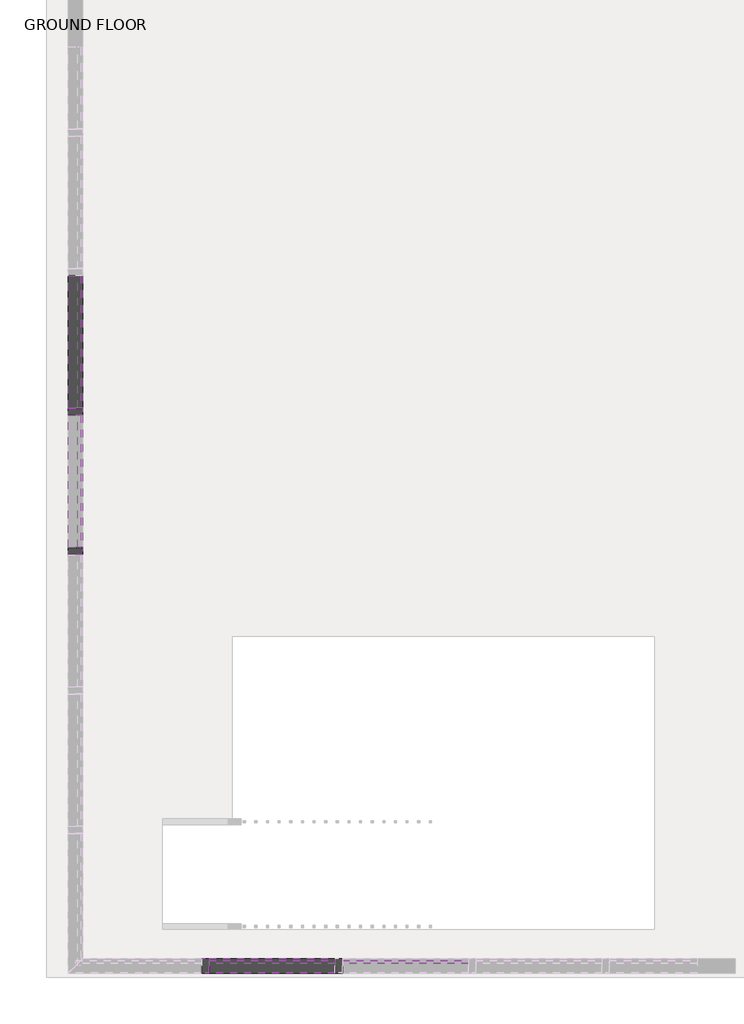
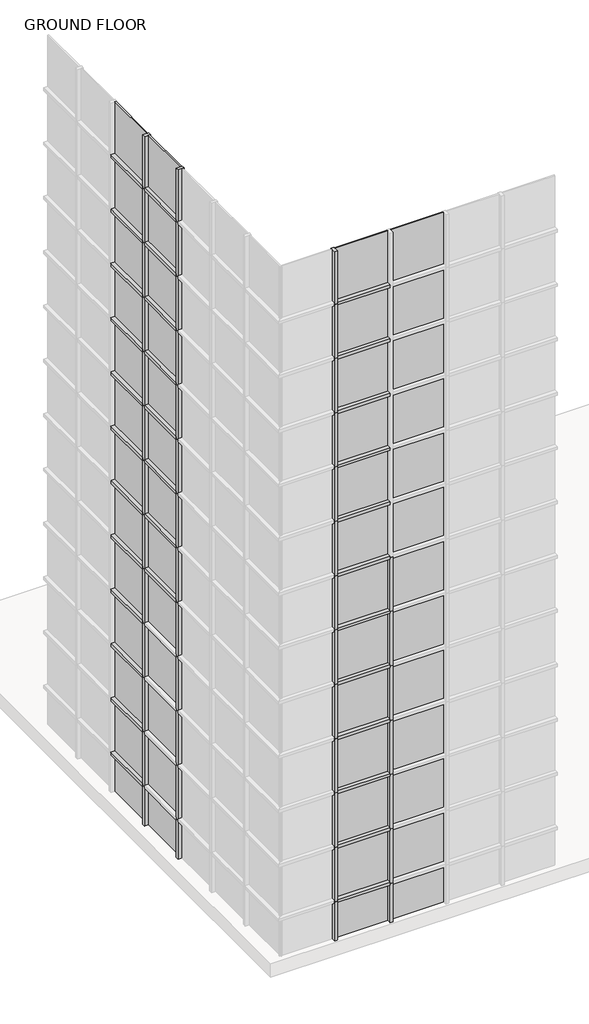
# One storey, part 2 of 16: 78 members, 52 plates.
"""IFC4 building model written with IfcOpenShell, lengths in millimetres."""

from ifc_helpers import new_model, si_unit, origin, place, context, project, spatial, transform, mapped, element, save
from components import member_d518c94e, member_b860638c, member_31fee25f, member_49b1bc66, system_panel_glazed_5cba32e5, system_panel_glazed_49652e9e

model = new_model("IFC4")

# Units and contexts
model_context = context("Model", 3, world=origin())
ifc_project = project(units=[si_unit("LENGTHUNIT", "METRE", prefix="MILLI")], contexts=[model_context])

# Site, building, storey
site = spatial("IfcSite", under=ifc_project)
building = spatial("IfcBuilding", under=site)
storey = spatial("IfcBuildingStorey", under=building, Name="GROUND FLOOR", Elevation=0.0)

# Members
placement = place(None, origin())
member_shape = member_d518c94e(model_context)
element("IfcMember", 1, ObjectType="Rectangular Mullion : 2.5\" x 5\" rectangular", at=placement, inside=storey, context=model_context, shape_type="MappedRepresentation", body=[
    mapped(member_shape, transform((-6857.4632917, -5739.2238032, 1168.8884615), x_axis=(0.0, 0.0, 1.0), y_axis=(0.0, -1.0, 0.0), z_axis=(1.0, 0.0, 0.0))),
])
element("IfcMember", 2, ObjectType="Rectangular Mullion : 2.5\" x 5\" rectangular", at=placement, inside=storey, context=model_context, shape_type="MappedRepresentation", body=[
    mapped(member_shape, transform((-6857.4632917, -5739.2238032, 2369.5269231), x_axis=(0.0, 0.0, 1.0), y_axis=(0.0, -1.0, 0.0), z_axis=(1.0, 0.0, 0.0))),
])
element("IfcMember", 3, ObjectType="Rectangular Mullion : 2.5\" x 5\" rectangular", at=placement, inside=storey, context=model_context, shape_type="MappedRepresentation", body=[
    mapped(member_shape, transform((-6857.4632917, -5739.2238032, 3570.1653846), x_axis=(0.0, 0.0, 1.0), y_axis=(0.0, -1.0, 0.0), z_axis=(1.0, 0.0, 0.0))),
])
element("IfcMember", 4, ObjectType="Rectangular Mullion : 2.5\" x 5\" rectangular", at=placement, inside=storey, context=model_context, shape_type="MappedRepresentation", body=[
    mapped(member_shape, transform((-6857.4632917, -5739.2238032, 4770.8038462), x_axis=(0.0, 0.0, 1.0), y_axis=(0.0, -1.0, 0.0), z_axis=(1.0, 0.0, 0.0))),
])
element("IfcMember", 5, ObjectType="Rectangular Mullion : 2.5\" x 5\" rectangular", at=placement, inside=storey, context=model_context, shape_type="MappedRepresentation", body=[
    mapped(member_shape, transform((-6857.4632917, -5739.2238032, 5971.4423077), x_axis=(0.0, 0.0, 1.0), y_axis=(0.0, -1.0, 0.0), z_axis=(1.0, 0.0, 0.0))),
])
element("IfcMember", 6, ObjectType="Rectangular Mullion : 2.5\" x 5\" rectangular", at=placement, inside=storey, context=model_context, shape_type="MappedRepresentation", body=[
    mapped(member_shape, transform((-6857.4632917, -5739.2238032, 7172.0807692), x_axis=(0.0, 0.0, 1.0), y_axis=(0.0, -1.0, 0.0), z_axis=(1.0, 0.0, 0.0))),
])
element("IfcMember", 7, ObjectType="Rectangular Mullion : 2.5\" x 5\" rectangular", at=placement, inside=storey, context=model_context, shape_type="MappedRepresentation", body=[
    mapped(member_shape, transform((-6857.4632917, -5739.2238032, 8372.7192308), x_axis=(0.0, 0.0, 1.0), y_axis=(0.0, -1.0, 0.0), z_axis=(1.0, 0.0, 0.0))),
])
element("IfcMember", 8, ObjectType="Rectangular Mullion : 2.5\" x 5\" rectangular", at=placement, inside=storey, context=model_context, shape_type="MappedRepresentation", body=[
    mapped(member_shape, transform((-6857.4632917, -5739.2238032, 9573.3576923), x_axis=(0.0, 0.0, 1.0), y_axis=(0.0, -1.0, 0.0), z_axis=(1.0, 0.0, 0.0))),
])
element("IfcMember", 9, ObjectType="Rectangular Mullion : 2.5\" x 5\" rectangular", at=placement, inside=storey, context=model_context, shape_type="MappedRepresentation", body=[
    mapped(member_shape, transform((-6857.4632917, -5739.2238032, 10773.9961538), x_axis=(0.0, 0.0, 1.0), y_axis=(0.0, -1.0, 0.0), z_axis=(1.0, 0.0, 0.0))),
])
element("IfcMember", 10, ObjectType="Rectangular Mullion : 2.5\" x 5\" rectangular", at=placement, inside=storey, context=model_context, shape_type="MappedRepresentation", body=[
    mapped(member_shape, transform((-6857.4632917, -5739.2238032, 11974.6346154), x_axis=(0.0, 0.0, 1.0), y_axis=(0.0, -1.0, 0.0), z_axis=(1.0, 0.0, 0.0))),
])
element("IfcMember", 11, ObjectType="Rectangular Mullion : 2.5\" x 5\" rectangular", at=placement, inside=storey, context=model_context, shape_type="MappedRepresentation", body=[
    mapped(member_shape, transform((-6857.4632917, -5739.2238032, 13175.2730769), x_axis=(0.0, 0.0, 1.0), y_axis=(0.0, -1.0, 0.0), z_axis=(1.0, 0.0, 0.0))),
])
element("IfcMember", 12, ObjectType="Rectangular Mullion : 2.5\" x 5\" rectangular", at=placement, inside=storey, context=model_context, shape_type="MappedRepresentation", body=[
    mapped(member_shape, transform((-6857.4632917, -5739.2238032, 14375.9115385), x_axis=(0.0, 0.0, 1.0), y_axis=(0.0, -1.0, 0.0), z_axis=(1.0, 0.0, 0.0))),
])
member_2_shape = member_b860638c(model_context)
element("IfcMember", 13, ObjectType="Rectangular Mullion : 2.5\" x 5\" rectangular", at=placement, inside=storey, context=model_context, shape_type="MappedRepresentation", body=[
    mapped(member_2_shape, transform((-7991.1825224, -5739.2238032, 0.0), x_axis=(1.0, 0.0, 0.0), y_axis=(0.0, -1.0, 0.0), z_axis=(0.0, 0.0, -1.0))),
])
element("IfcMember", 14, ObjectType="Rectangular Mullion : 2.5\" x 5\" rectangular", at=placement, inside=storey, context=model_context, shape_type="MappedRepresentation", body=[
    mapped(member_2_shape, transform((-6825.7132917, -5739.2238032, 0.0), x_axis=(1.0, 0.0, 0.0), y_axis=(0.0, -1.0, 0.0), z_axis=(0.0, 0.0, -1.0))),
])
element("IfcMember", 15, ObjectType="Rectangular Mullion : 2.5\" x 5\" rectangular", at=placement, inside=storey, context=model_context, shape_type="MappedRepresentation", body=[
    mapped(member_2_shape, transform((-9124.9017534, -901.7938032, 0.0), x_axis=(0.0, -1.0, 0.0), y_axis=(-1.0, 0.0, 0.0), z_axis=(0.0, 0.0, -1.0))),
])
element("IfcMember", 16, ObjectType="Rectangular Mullion : 2.5\" x 5\" rectangular", at=placement, inside=storey, context=model_context, shape_type="MappedRepresentation", body=[
    mapped(member_2_shape, transform((-9124.9017534, -2119.0888031, 0.0), x_axis=(0.0, -1.0, 0.0), y_axis=(-1.0, 0.0, 0.0), z_axis=(0.0, 0.0, -1.0))),
])
member_3_shape = member_31fee25f(model_context)
element("IfcMember", 17, ObjectType="Rectangular Mullion : 2.5\" x 5\" rectangular", at=placement, inside=storey, context=model_context, shape_type="MappedRepresentation", body=[
    mapped(member_3_shape, transform((-7991.1825224, -5739.2238032, 1168.8884615), x_axis=(1.0, 0.0, 0.0), y_axis=(0.0, -1.0, 0.0), z_axis=(0.0, 0.0, -1.0))),
])
element("IfcMember", 18, ObjectType="Rectangular Mullion : 2.5\" x 5\" rectangular", at=placement, inside=storey, context=model_context, shape_type="MappedRepresentation", body=[
    mapped(member_3_shape, transform((-6825.7132917, -5739.2238032, 1168.8884615), x_axis=(1.0, 0.0, 0.0), y_axis=(0.0, -1.0, 0.0), z_axis=(0.0, 0.0, -1.0))),
])
element("IfcMember", 19, ObjectType="Rectangular Mullion : 2.5\" x 5\" rectangular", at=placement, inside=storey, context=model_context, shape_type="MappedRepresentation", body=[
    mapped(member_3_shape, transform((-7991.1825224, -5739.2238032, 2369.5269231), x_axis=(1.0, 0.0, 0.0), y_axis=(0.0, -1.0, 0.0), z_axis=(0.0, 0.0, -1.0))),
])
element("IfcMember", 20, ObjectType="Rectangular Mullion : 2.5\" x 5\" rectangular", at=placement, inside=storey, context=model_context, shape_type="MappedRepresentation", body=[
    mapped(member_3_shape, transform((-6825.7132917, -5739.2238032, 2369.5269231), x_axis=(1.0, 0.0, 0.0), y_axis=(0.0, -1.0, 0.0), z_axis=(0.0, 0.0, -1.0))),
])
element("IfcMember", 21, ObjectType="Rectangular Mullion : 2.5\" x 5\" rectangular", at=placement, inside=storey, context=model_context, shape_type="MappedRepresentation", body=[
    mapped(member_3_shape, transform((-7991.1825224, -5739.2238032, 3570.1653846), x_axis=(1.0, 0.0, 0.0), y_axis=(0.0, -1.0, 0.0), z_axis=(0.0, 0.0, -1.0))),
])
element("IfcMember", 22, ObjectType="Rectangular Mullion : 2.5\" x 5\" rectangular", at=placement, inside=storey, context=model_context, shape_type="MappedRepresentation", body=[
    mapped(member_3_shape, transform((-6825.7132917, -5739.2238032, 3570.1653846), x_axis=(1.0, 0.0, 0.0), y_axis=(0.0, -1.0, 0.0), z_axis=(0.0, 0.0, -1.0))),
])
element("IfcMember", 23, ObjectType="Rectangular Mullion : 2.5\" x 5\" rectangular", at=placement, inside=storey, context=model_context, shape_type="MappedRepresentation", body=[
    mapped(member_3_shape, transform((-7991.1825224, -5739.2238032, 4770.8038462), x_axis=(1.0, 0.0, 0.0), y_axis=(0.0, -1.0, 0.0), z_axis=(0.0, 0.0, -1.0))),
])
element("IfcMember", 24, ObjectType="Rectangular Mullion : 2.5\" x 5\" rectangular", at=placement, inside=storey, context=model_context, shape_type="MappedRepresentation", body=[
    mapped(member_3_shape, transform((-6825.7132917, -5739.2238032, 4770.8038462), x_axis=(1.0, 0.0, 0.0), y_axis=(0.0, -1.0, 0.0), z_axis=(0.0, 0.0, -1.0))),
])
element("IfcMember", 25, ObjectType="Rectangular Mullion : 2.5\" x 5\" rectangular", at=placement, inside=storey, context=model_context, shape_type="MappedRepresentation", body=[
    mapped(member_3_shape, transform((-7991.1825224, -5739.2238032, 5971.4423077), x_axis=(1.0, 0.0, 0.0), y_axis=(0.0, -1.0, 0.0), z_axis=(0.0, 0.0, -1.0))),
])
element("IfcMember", 26, ObjectType="Rectangular Mullion : 2.5\" x 5\" rectangular", at=placement, inside=storey, context=model_context, shape_type="MappedRepresentation", body=[
    mapped(member_3_shape, transform((-6825.7132917, -5739.2238032, 5971.4423077), x_axis=(1.0, 0.0, 0.0), y_axis=(0.0, -1.0, 0.0), z_axis=(0.0, 0.0, -1.0))),
])
element("IfcMember", 27, ObjectType="Rectangular Mullion : 2.5\" x 5\" rectangular", at=placement, inside=storey, context=model_context, shape_type="MappedRepresentation", body=[
    mapped(member_3_shape, transform((-7991.1825224, -5739.2238032, 7172.0807692), x_axis=(1.0, 0.0, 0.0), y_axis=(0.0, -1.0, 0.0), z_axis=(0.0, 0.0, -1.0))),
])
element("IfcMember", 28, ObjectType="Rectangular Mullion : 2.5\" x 5\" rectangular", at=placement, inside=storey, context=model_context, shape_type="MappedRepresentation", body=[
    mapped(member_3_shape, transform((-6825.7132917, -5739.2238032, 7172.0807692), x_axis=(1.0, 0.0, 0.0), y_axis=(0.0, -1.0, 0.0), z_axis=(0.0, 0.0, -1.0))),
])
element("IfcMember", 29, ObjectType="Rectangular Mullion : 2.5\" x 5\" rectangular", at=placement, inside=storey, context=model_context, shape_type="MappedRepresentation", body=[
    mapped(member_3_shape, transform((-7991.1825224, -5739.2238032, 8372.7192308), x_axis=(1.0, 0.0, 0.0), y_axis=(0.0, -1.0, 0.0), z_axis=(0.0, 0.0, -1.0))),
])
element("IfcMember", 30, ObjectType="Rectangular Mullion : 2.5\" x 5\" rectangular", at=placement, inside=storey, context=model_context, shape_type="MappedRepresentation", body=[
    mapped(member_3_shape, transform((-7991.1825224, -5739.2238032, 9573.3576923), x_axis=(1.0, 0.0, 0.0), y_axis=(0.0, -1.0, 0.0), z_axis=(0.0, 0.0, -1.0))),
])
element("IfcMember", 31, ObjectType="Rectangular Mullion : 2.5\" x 5\" rectangular", at=placement, inside=storey, context=model_context, shape_type="MappedRepresentation", body=[
    mapped(member_3_shape, transform((-7991.1825224, -5739.2238032, 10773.9961538), x_axis=(1.0, 0.0, 0.0), y_axis=(0.0, -1.0, 0.0), z_axis=(0.0, 0.0, -1.0))),
])
element("IfcMember", 32, ObjectType="Rectangular Mullion : 2.5\" x 5\" rectangular", at=placement, inside=storey, context=model_context, shape_type="MappedRepresentation", body=[
    mapped(member_3_shape, transform((-7991.1825224, -5739.2238032, 11974.6346154), x_axis=(1.0, 0.0, 0.0), y_axis=(0.0, -1.0, 0.0), z_axis=(0.0, 0.0, -1.0))),
])
element("IfcMember", 33, ObjectType="Rectangular Mullion : 2.5\" x 5\" rectangular", at=placement, inside=storey, context=model_context, shape_type="MappedRepresentation", body=[
    mapped(member_3_shape, transform((-7991.1825224, -5739.2238032, 13175.2730769), x_axis=(1.0, 0.0, 0.0), y_axis=(0.0, -1.0, 0.0), z_axis=(0.0, 0.0, -1.0))),
])
element("IfcMember", 34, ObjectType="Rectangular Mullion : 2.5\" x 5\" rectangular", at=placement, inside=storey, context=model_context, shape_type="MappedRepresentation", body=[
    mapped(member_3_shape, transform((-9124.9017534, -901.7938032, 1168.8884615), x_axis=(0.0, -1.0, 0.0), y_axis=(-1.0, 0.0, 0.0), z_axis=(0.0, 0.0, -1.0))),
])
element("IfcMember", 35, ObjectType="Rectangular Mullion : 2.5\" x 5\" rectangular", at=placement, inside=storey, context=model_context, shape_type="MappedRepresentation", body=[
    mapped(member_3_shape, transform((-9124.9017534, -2119.0888031, 1168.8884615), x_axis=(0.0, -1.0, 0.0), y_axis=(-1.0, 0.0, 0.0), z_axis=(0.0, 0.0, -1.0))),
])
element("IfcMember", 36, ObjectType="Rectangular Mullion : 2.5\" x 5\" rectangular", at=placement, inside=storey, context=model_context, shape_type="MappedRepresentation", body=[
    mapped(member_3_shape, transform((-9124.9017534, -901.7938032, 2369.5269231), x_axis=(0.0, -1.0, 0.0), y_axis=(-1.0, 0.0, 0.0), z_axis=(0.0, 0.0, -1.0))),
])
element("IfcMember", 37, ObjectType="Rectangular Mullion : 2.5\" x 5\" rectangular", at=placement, inside=storey, context=model_context, shape_type="MappedRepresentation", body=[
    mapped(member_3_shape, transform((-9124.9017534, -2119.0888031, 2369.5269231), x_axis=(0.0, -1.0, 0.0), y_axis=(-1.0, 0.0, 0.0), z_axis=(0.0, 0.0, -1.0))),
])
element("IfcMember", 38, ObjectType="Rectangular Mullion : 2.5\" x 5\" rectangular", at=placement, inside=storey, context=model_context, shape_type="MappedRepresentation", body=[
    mapped(member_3_shape, transform((-9124.9017534, -901.7938032, 3570.1653846), x_axis=(0.0, -1.0, 0.0), y_axis=(-1.0, 0.0, 0.0), z_axis=(0.0, 0.0, -1.0))),
])
element("IfcMember", 39, ObjectType="Rectangular Mullion : 2.5\" x 5\" rectangular", at=placement, inside=storey, context=model_context, shape_type="MappedRepresentation", body=[
    mapped(member_3_shape, transform((-9124.9017534, -2119.0888031, 3570.1653846), x_axis=(0.0, -1.0, 0.0), y_axis=(-1.0, 0.0, 0.0), z_axis=(0.0, 0.0, -1.0))),
])
element("IfcMember", 40, ObjectType="Rectangular Mullion : 2.5\" x 5\" rectangular", at=placement, inside=storey, context=model_context, shape_type="MappedRepresentation", body=[
    mapped(member_3_shape, transform((-9124.9017534, -901.7938032, 4770.8038462), x_axis=(0.0, -1.0, 0.0), y_axis=(-1.0, 0.0, 0.0), z_axis=(0.0, 0.0, -1.0))),
])
element("IfcMember", 41, ObjectType="Rectangular Mullion : 2.5\" x 5\" rectangular", at=placement, inside=storey, context=model_context, shape_type="MappedRepresentation", body=[
    mapped(member_3_shape, transform((-9124.9017534, -2119.0888031, 4770.8038462), x_axis=(0.0, -1.0, 0.0), y_axis=(-1.0, 0.0, 0.0), z_axis=(0.0, 0.0, -1.0))),
])
element("IfcMember", 42, ObjectType="Rectangular Mullion : 2.5\" x 5\" rectangular", at=placement, inside=storey, context=model_context, shape_type="MappedRepresentation", body=[
    mapped(member_3_shape, transform((-9124.9017534, -901.7938032, 5971.4423077), x_axis=(0.0, -1.0, 0.0), y_axis=(-1.0, 0.0, 0.0), z_axis=(0.0, 0.0, -1.0))),
])
element("IfcMember", 43, ObjectType="Rectangular Mullion : 2.5\" x 5\" rectangular", at=placement, inside=storey, context=model_context, shape_type="MappedRepresentation", body=[
    mapped(member_3_shape, transform((-9124.9017534, -2119.0888031, 5971.4423077), x_axis=(0.0, -1.0, 0.0), y_axis=(-1.0, 0.0, 0.0), z_axis=(0.0, 0.0, -1.0))),
])
element("IfcMember", 44, ObjectType="Rectangular Mullion : 2.5\" x 5\" rectangular", at=placement, inside=storey, context=model_context, shape_type="MappedRepresentation", body=[
    mapped(member_3_shape, transform((-9124.9017534, -901.7938032, 7172.0807692), x_axis=(0.0, -1.0, 0.0), y_axis=(-1.0, 0.0, 0.0), z_axis=(0.0, 0.0, -1.0))),
])
element("IfcMember", 45, ObjectType="Rectangular Mullion : 2.5\" x 5\" rectangular", at=placement, inside=storey, context=model_context, shape_type="MappedRepresentation", body=[
    mapped(member_3_shape, transform((-9124.9017534, -2119.0888031, 7172.0807692), x_axis=(0.0, -1.0, 0.0), y_axis=(-1.0, 0.0, 0.0), z_axis=(0.0, 0.0, -1.0))),
])
element("IfcMember", 46, ObjectType="Rectangular Mullion : 2.5\" x 5\" rectangular", at=placement, inside=storey, context=model_context, shape_type="MappedRepresentation", body=[
    mapped(member_3_shape, transform((-9124.9017534, -901.7938032, 8372.7192308), x_axis=(0.0, -1.0, 0.0), y_axis=(-1.0, 0.0, 0.0), z_axis=(0.0, 0.0, -1.0))),
])
element("IfcMember", 47, ObjectType="Rectangular Mullion : 2.5\" x 5\" rectangular", at=placement, inside=storey, context=model_context, shape_type="MappedRepresentation", body=[
    mapped(member_3_shape, transform((-9124.9017534, -2119.0888031, 8372.7192308), x_axis=(0.0, -1.0, 0.0), y_axis=(-1.0, 0.0, 0.0), z_axis=(0.0, 0.0, -1.0))),
])
element("IfcMember", 48, ObjectType="Rectangular Mullion : 2.5\" x 5\" rectangular", at=placement, inside=storey, context=model_context, shape_type="MappedRepresentation", body=[
    mapped(member_3_shape, transform((-9124.9017534, -901.7938032, 9573.3576923), x_axis=(0.0, -1.0, 0.0), y_axis=(-1.0, 0.0, 0.0), z_axis=(0.0, 0.0, -1.0))),
])
element("IfcMember", 49, ObjectType="Rectangular Mullion : 2.5\" x 5\" rectangular", at=placement, inside=storey, context=model_context, shape_type="MappedRepresentation", body=[
    mapped(member_3_shape, transform((-9124.9017534, -2119.0888031, 9573.3576923), x_axis=(0.0, -1.0, 0.0), y_axis=(-1.0, 0.0, 0.0), z_axis=(0.0, 0.0, -1.0))),
])
element("IfcMember", 50, ObjectType="Rectangular Mullion : 2.5\" x 5\" rectangular", at=placement, inside=storey, context=model_context, shape_type="MappedRepresentation", body=[
    mapped(member_3_shape, transform((-9124.9017534, -901.7938032, 10773.9961538), x_axis=(0.0, -1.0, 0.0), y_axis=(-1.0, 0.0, 0.0), z_axis=(0.0, 0.0, -1.0))),
])
element("IfcMember", 51, ObjectType="Rectangular Mullion : 2.5\" x 5\" rectangular", at=placement, inside=storey, context=model_context, shape_type="MappedRepresentation", body=[
    mapped(member_3_shape, transform((-9124.9017534, -2119.0888031, 10773.9961538), x_axis=(0.0, -1.0, 0.0), y_axis=(-1.0, 0.0, 0.0), z_axis=(0.0, 0.0, -1.0))),
])
element("IfcMember", 52, ObjectType="Rectangular Mullion : 2.5\" x 5\" rectangular", at=placement, inside=storey, context=model_context, shape_type="MappedRepresentation", body=[
    mapped(member_3_shape, transform((-9124.9017534, -901.7938032, 11974.6346154), x_axis=(0.0, -1.0, 0.0), y_axis=(-1.0, 0.0, 0.0), z_axis=(0.0, 0.0, -1.0))),
])
element("IfcMember", 53, ObjectType="Rectangular Mullion : 2.5\" x 5\" rectangular", at=placement, inside=storey, context=model_context, shape_type="MappedRepresentation", body=[
    mapped(member_3_shape, transform((-9124.9017534, -2119.0888031, 11974.6346154), x_axis=(0.0, -1.0, 0.0), y_axis=(-1.0, 0.0, 0.0), z_axis=(0.0, 0.0, -1.0))),
])
element("IfcMember", 54, ObjectType="Rectangular Mullion : 2.5\" x 5\" rectangular", at=placement, inside=storey, context=model_context, shape_type="MappedRepresentation", body=[
    mapped(member_3_shape, transform((-9124.9017534, -901.7938032, 13175.2730769), x_axis=(0.0, -1.0, 0.0), y_axis=(-1.0, 0.0, 0.0), z_axis=(0.0, 0.0, -1.0))),
])
element("IfcMember", 55, ObjectType="Rectangular Mullion : 2.5\" x 5\" rectangular", at=placement, inside=storey, context=model_context, shape_type="MappedRepresentation", body=[
    mapped(member_3_shape, transform((-9124.9017534, -2119.0888031, 13175.2730769), x_axis=(0.0, -1.0, 0.0), y_axis=(-1.0, 0.0, 0.0), z_axis=(0.0, 0.0, -1.0))),
])
element("IfcMember", 56, ObjectType="Rectangular Mullion : 2.5\" x 5\" rectangular", at=placement, inside=storey, context=model_context, shape_type="MappedRepresentation", body=[
    mapped(member_2_shape, transform((-7991.1825224, -5739.2238032, 14375.9115385), x_axis=(1.0, 0.0, 0.0), y_axis=(0.0, -1.0, 0.0), z_axis=(0.0, 0.0, -1.0))),
])
element("IfcMember", 57, ObjectType="Rectangular Mullion : 2.5\" x 5\" rectangular", at=placement, inside=storey, context=model_context, shape_type="MappedRepresentation", body=[
    mapped(member_2_shape, transform((-9124.9017534, -901.7938032, 14375.9115385), x_axis=(0.0, -1.0, 0.0), y_axis=(-1.0, 0.0, 0.0), z_axis=(0.0, 0.0, -1.0))),
])
element("IfcMember", 58, ObjectType="Rectangular Mullion : 2.5\" x 5\" rectangular", at=placement, inside=storey, context=model_context, shape_type="MappedRepresentation", body=[
    mapped(member_2_shape, transform((-9124.9017534, -2119.0888031, 14375.9115385), x_axis=(0.0, -1.0, 0.0), y_axis=(-1.0, 0.0, 0.0), z_axis=(0.0, 0.0, -1.0))),
])
member_4_shape = member_49b1bc66(model_context)
element("IfcMember", 59, ObjectType="Rectangular Mullion : 2.5\" x 5\" rectangular", at=placement, inside=storey, context=model_context, shape_type="MappedRepresentation", body=[
    mapped(member_4_shape, transform((-9124.9017534, -870.0438032, 1168.8884615), x_axis=(0.0, 0.0, 1.0), y_axis=(-1.0, 0.0, 0.0), z_axis=(0.0, -1.0, 0.0))),
])
element("IfcMember", 60, ObjectType="Rectangular Mullion : 2.5\" x 5\" rectangular", at=placement, inside=storey, context=model_context, shape_type="MappedRepresentation", body=[
    mapped(member_4_shape, transform((-9124.9017534, -870.0438032, 2369.5269231), x_axis=(0.0, 0.0, 1.0), y_axis=(-1.0, 0.0, 0.0), z_axis=(0.0, -1.0, 0.0))),
])
element("IfcMember", 61, ObjectType="Rectangular Mullion : 2.5\" x 5\" rectangular", at=placement, inside=storey, context=model_context, shape_type="MappedRepresentation", body=[
    mapped(member_4_shape, transform((-9124.9017534, -870.0438032, 3570.1653846), x_axis=(0.0, 0.0, 1.0), y_axis=(-1.0, 0.0, 0.0), z_axis=(0.0, -1.0, 0.0))),
])
element("IfcMember", 62, ObjectType="Rectangular Mullion : 2.5\" x 5\" rectangular", at=placement, inside=storey, context=model_context, shape_type="MappedRepresentation", body=[
    mapped(member_4_shape, transform((-9124.9017534, -870.0438032, 4770.8038462), x_axis=(0.0, 0.0, 1.0), y_axis=(-1.0, 0.0, 0.0), z_axis=(0.0, -1.0, 0.0))),
])
element("IfcMember", 63, ObjectType="Rectangular Mullion : 2.5\" x 5\" rectangular", at=placement, inside=storey, context=model_context, shape_type="MappedRepresentation", body=[
    mapped(member_4_shape, transform((-9124.9017534, -870.0438032, 5971.4423077), x_axis=(0.0, 0.0, 1.0), y_axis=(-1.0, 0.0, 0.0), z_axis=(0.0, -1.0, 0.0))),
])
element("IfcMember", 64, ObjectType="Rectangular Mullion : 2.5\" x 5\" rectangular", at=placement, inside=storey, context=model_context, shape_type="MappedRepresentation", body=[
    mapped(member_4_shape, transform((-9124.9017534, -2087.3388031, 5971.4423077), x_axis=(0.0, 0.0, 1.0), y_axis=(-1.0, 0.0, 0.0), z_axis=(0.0, -1.0, 0.0))),
])
element("IfcMember", 65, ObjectType="Rectangular Mullion : 2.5\" x 5\" rectangular", at=placement, inside=storey, context=model_context, shape_type="MappedRepresentation", body=[
    mapped(member_4_shape, transform((-9124.9017534, -870.0438032, 7172.0807692), x_axis=(0.0, 0.0, 1.0), y_axis=(-1.0, 0.0, 0.0), z_axis=(0.0, -1.0, 0.0))),
])
element("IfcMember", 66, ObjectType="Rectangular Mullion : 2.5\" x 5\" rectangular", at=placement, inside=storey, context=model_context, shape_type="MappedRepresentation", body=[
    mapped(member_4_shape, transform((-9124.9017534, -2087.3388031, 7172.0807692), x_axis=(0.0, 0.0, 1.0), y_axis=(-1.0, 0.0, 0.0), z_axis=(0.0, -1.0, 0.0))),
])
element("IfcMember", 67, ObjectType="Rectangular Mullion : 2.5\" x 5\" rectangular", at=placement, inside=storey, context=model_context, shape_type="MappedRepresentation", body=[
    mapped(member_4_shape, transform((-9124.9017534, -870.0438032, 8372.7192308), x_axis=(0.0, 0.0, 1.0), y_axis=(-1.0, 0.0, 0.0), z_axis=(0.0, -1.0, 0.0))),
])
element("IfcMember", 68, ObjectType="Rectangular Mullion : 2.5\" x 5\" rectangular", at=placement, inside=storey, context=model_context, shape_type="MappedRepresentation", body=[
    mapped(member_4_shape, transform((-9124.9017534, -2087.3388031, 8372.7192308), x_axis=(0.0, 0.0, 1.0), y_axis=(-1.0, 0.0, 0.0), z_axis=(0.0, -1.0, 0.0))),
])
element("IfcMember", 69, ObjectType="Rectangular Mullion : 2.5\" x 5\" rectangular", at=placement, inside=storey, context=model_context, shape_type="MappedRepresentation", body=[
    mapped(member_4_shape, transform((-9124.9017534, -870.0438032, 9573.3576923), x_axis=(0.0, 0.0, 1.0), y_axis=(-1.0, 0.0, 0.0), z_axis=(0.0, -1.0, 0.0))),
])
element("IfcMember", 70, ObjectType="Rectangular Mullion : 2.5\" x 5\" rectangular", at=placement, inside=storey, context=model_context, shape_type="MappedRepresentation", body=[
    mapped(member_4_shape, transform((-9124.9017534, -2087.3388031, 9573.3576923), x_axis=(0.0, 0.0, 1.0), y_axis=(-1.0, 0.0, 0.0), z_axis=(0.0, -1.0, 0.0))),
])
element("IfcMember", 71, ObjectType="Rectangular Mullion : 2.5\" x 5\" rectangular", at=placement, inside=storey, context=model_context, shape_type="MappedRepresentation", body=[
    mapped(member_4_shape, transform((-9124.9017534, -870.0438032, 10773.9961538), x_axis=(0.0, 0.0, 1.0), y_axis=(-1.0, 0.0, 0.0), z_axis=(0.0, -1.0, 0.0))),
])
element("IfcMember", 72, ObjectType="Rectangular Mullion : 2.5\" x 5\" rectangular", at=placement, inside=storey, context=model_context, shape_type="MappedRepresentation", body=[
    mapped(member_4_shape, transform((-9124.9017534, -2087.3388031, 10773.9961538), x_axis=(0.0, 0.0, 1.0), y_axis=(-1.0, 0.0, 0.0), z_axis=(0.0, -1.0, 0.0))),
])
element("IfcMember", 73, ObjectType="Rectangular Mullion : 2.5\" x 5\" rectangular", at=placement, inside=storey, context=model_context, shape_type="MappedRepresentation", body=[
    mapped(member_4_shape, transform((-9124.9017534, -870.0438032, 11974.6346154), x_axis=(0.0, 0.0, 1.0), y_axis=(-1.0, 0.0, 0.0), z_axis=(0.0, -1.0, 0.0))),
])
element("IfcMember", 74, ObjectType="Rectangular Mullion : 2.5\" x 5\" rectangular", at=placement, inside=storey, context=model_context, shape_type="MappedRepresentation", body=[
    mapped(member_4_shape, transform((-9124.9017534, -2087.3388031, 11974.6346154), x_axis=(0.0, 0.0, 1.0), y_axis=(-1.0, 0.0, 0.0), z_axis=(0.0, -1.0, 0.0))),
])
element("IfcMember", 75, ObjectType="Rectangular Mullion : 2.5\" x 5\" rectangular", at=placement, inside=storey, context=model_context, shape_type="MappedRepresentation", body=[
    mapped(member_4_shape, transform((-9124.9017534, -870.0438032, 13175.2730769), x_axis=(0.0, 0.0, 1.0), y_axis=(-1.0, 0.0, 0.0), z_axis=(0.0, -1.0, 0.0))),
])
element("IfcMember", 76, ObjectType="Rectangular Mullion : 2.5\" x 5\" rectangular", at=placement, inside=storey, context=model_context, shape_type="MappedRepresentation", body=[
    mapped(member_4_shape, transform((-9124.9017534, -2087.3388031, 13175.2730769), x_axis=(0.0, 0.0, 1.0), y_axis=(-1.0, 0.0, 0.0), z_axis=(0.0, -1.0, 0.0))),
])
element("IfcMember", 77, ObjectType="Rectangular Mullion : 2.5\" x 5\" rectangular", at=placement, inside=storey, context=model_context, shape_type="MappedRepresentation", body=[
    mapped(member_4_shape, transform((-9124.9017534, -870.0438032, 14375.9115385), x_axis=(0.0, 0.0, 1.0), y_axis=(-1.0, 0.0, 0.0), z_axis=(0.0, -1.0, 0.0))),
])
element("IfcMember", 78, ObjectType="Rectangular Mullion : 2.5\" x 5\" rectangular", at=placement, inside=storey, context=model_context, shape_type="MappedRepresentation", body=[
    mapped(member_4_shape, transform((-9124.9017534, -2087.3388031, 14375.9115385), x_axis=(0.0, 0.0, 1.0), y_axis=(-1.0, 0.0, 0.0), z_axis=(0.0, -1.0, 0.0))),
])

# Plates
system_panel_glazed_shape = system_panel_glazed_5cba32e5(model_context)
element("IfcPlate", 79, ObjectType="System Panel : Glazed", at=placement, inside=storey, context=model_context, shape_type="MappedRepresentation", body=[
    mapped(system_panel_glazed_shape, transform((-7408.447907, -5739.2238032, 0.0), x_axis=(1.0, 0.0, 0.0), y_axis=(0.0, 1.0, 0.0), z_axis=(0.0, 0.0, 1.0))),
])
element("IfcPlate", 80, ObjectType="System Panel : Glazed", at=placement, inside=storey, context=model_context, shape_type="MappedRepresentation", body=[
    mapped(system_panel_glazed_shape, transform((-6242.9786763, -5739.2238032, 0.0), x_axis=(1.0, 0.0, 0.0), y_axis=(0.0, 1.0, 0.0), z_axis=(0.0, 0.0, 1.0))),
])
element("IfcPlate", 81, ObjectType="System Panel : Glazed", at=placement, inside=storey, context=model_context, shape_type="MappedRepresentation", body=[
    mapped(system_panel_glazed_shape, transform((-7408.447907, -5739.2238032, 1200.6384615), x_axis=(1.0, 0.0, 0.0), y_axis=(0.0, 1.0, 0.0), z_axis=(0.0, 0.0, 1.0))),
])
element("IfcPlate", 82, ObjectType="System Panel : Glazed", at=placement, inside=storey, context=model_context, shape_type="MappedRepresentation", body=[
    mapped(system_panel_glazed_shape, transform((-6242.9786763, -5739.2238032, 1200.6384615), x_axis=(1.0, 0.0, 0.0), y_axis=(0.0, 1.0, 0.0), z_axis=(0.0, 0.0, 1.0))),
])
element("IfcPlate", 83, ObjectType="System Panel : Glazed", at=placement, inside=storey, context=model_context, shape_type="MappedRepresentation", body=[
    mapped(system_panel_glazed_shape, transform((-7408.447907, -5739.2238032, 2401.2769231), x_axis=(1.0, 0.0, 0.0), y_axis=(0.0, 1.0, 0.0), z_axis=(0.0, 0.0, 1.0))),
])
element("IfcPlate", 84, ObjectType="System Panel : Glazed", at=placement, inside=storey, context=model_context, shape_type="MappedRepresentation", body=[
    mapped(system_panel_glazed_shape, transform((-6242.9786763, -5739.2238032, 2401.2769231), x_axis=(1.0, 0.0, 0.0), y_axis=(0.0, 1.0, 0.0), z_axis=(0.0, 0.0, 1.0))),
])
element("IfcPlate", 85, ObjectType="System Panel : Glazed", at=placement, inside=storey, context=model_context, shape_type="MappedRepresentation", body=[
    mapped(system_panel_glazed_shape, transform((-7408.447907, -5739.2238032, 3601.9153846), x_axis=(1.0, 0.0, 0.0), y_axis=(0.0, 1.0, 0.0), z_axis=(0.0, 0.0, 1.0))),
])
element("IfcPlate", 86, ObjectType="System Panel : Glazed", at=placement, inside=storey, context=model_context, shape_type="MappedRepresentation", body=[
    mapped(system_panel_glazed_shape, transform((-6242.9786763, -5739.2238032, 3601.9153846), x_axis=(1.0, 0.0, 0.0), y_axis=(0.0, 1.0, 0.0), z_axis=(0.0, 0.0, 1.0))),
])
element("IfcPlate", 87, ObjectType="System Panel : Glazed", at=placement, inside=storey, context=model_context, shape_type="MappedRepresentation", body=[
    mapped(system_panel_glazed_shape, transform((-7408.447907, -5739.2238032, 4802.5538462), x_axis=(1.0, 0.0, 0.0), y_axis=(0.0, 1.0, 0.0), z_axis=(0.0, 0.0, 1.0))),
])
element("IfcPlate", 88, ObjectType="System Panel : Glazed", at=placement, inside=storey, context=model_context, shape_type="MappedRepresentation", body=[
    mapped(system_panel_glazed_shape, transform((-6242.9786763, -5739.2238032, 4802.5538462), x_axis=(1.0, 0.0, 0.0), y_axis=(0.0, 1.0, 0.0), z_axis=(0.0, 0.0, 1.0))),
])
element("IfcPlate", 89, ObjectType="System Panel : Glazed", at=placement, inside=storey, context=model_context, shape_type="MappedRepresentation", body=[
    mapped(system_panel_glazed_shape, transform((-7408.447907, -5739.2238032, 6003.1923077), x_axis=(1.0, 0.0, 0.0), y_axis=(0.0, 1.0, 0.0), z_axis=(0.0, 0.0, 1.0))),
])
element("IfcPlate", 90, ObjectType="System Panel : Glazed", at=placement, inside=storey, context=model_context, shape_type="MappedRepresentation", body=[
    mapped(system_panel_glazed_shape, transform((-6242.9786763, -5739.2238032, 6003.1923077), x_axis=(1.0, 0.0, 0.0), y_axis=(0.0, 1.0, 0.0), z_axis=(0.0, 0.0, 1.0))),
])
element("IfcPlate", 91, ObjectType="System Panel : Glazed", at=placement, inside=storey, context=model_context, shape_type="MappedRepresentation", body=[
    mapped(system_panel_glazed_shape, transform((-7408.447907, -5739.2238032, 7203.8307692), x_axis=(1.0, 0.0, 0.0), y_axis=(0.0, 1.0, 0.0), z_axis=(0.0, 0.0, 1.0))),
])
element("IfcPlate", 92, ObjectType="System Panel : Glazed", at=placement, inside=storey, context=model_context, shape_type="MappedRepresentation", body=[
    mapped(system_panel_glazed_shape, transform((-6242.9786763, -5739.2238032, 7203.8307692), x_axis=(1.0, 0.0, 0.0), y_axis=(0.0, 1.0, 0.0), z_axis=(0.0, 0.0, 1.0))),
])
element("IfcPlate", 93, ObjectType="System Panel : Glazed", at=placement, inside=storey, context=model_context, shape_type="MappedRepresentation", body=[
    mapped(system_panel_glazed_shape, transform((-7408.447907, -5739.2238032, 8404.4692308), x_axis=(1.0, 0.0, 0.0), y_axis=(0.0, 1.0, 0.0), z_axis=(0.0, 0.0, 1.0))),
])
element("IfcPlate", 94, ObjectType="System Panel : Glazed", at=placement, inside=storey, context=model_context, shape_type="MappedRepresentation", body=[
    mapped(system_panel_glazed_shape, transform((-6242.9786763, -5739.2238032, 8404.4692308), x_axis=(1.0, 0.0, 0.0), y_axis=(0.0, 1.0, 0.0), z_axis=(0.0, 0.0, 1.0))),
])
element("IfcPlate", 95, ObjectType="System Panel : Glazed", at=placement, inside=storey, context=model_context, shape_type="MappedRepresentation", body=[
    mapped(system_panel_glazed_shape, transform((-7408.447907, -5739.2238032, 9605.1076923), x_axis=(1.0, 0.0, 0.0), y_axis=(0.0, 1.0, 0.0), z_axis=(0.0, 0.0, 1.0))),
])
element("IfcPlate", 96, ObjectType="System Panel : Glazed", at=placement, inside=storey, context=model_context, shape_type="MappedRepresentation", body=[
    mapped(system_panel_glazed_shape, transform((-6242.9786763, -5739.2238032, 9605.1076923), x_axis=(1.0, 0.0, 0.0), y_axis=(0.0, 1.0, 0.0), z_axis=(0.0, 0.0, 1.0))),
])
element("IfcPlate", 97, ObjectType="System Panel : Glazed", at=placement, inside=storey, context=model_context, shape_type="MappedRepresentation", body=[
    mapped(system_panel_glazed_shape, transform((-7408.447907, -5739.2238032, 10805.7461538), x_axis=(1.0, 0.0, 0.0), y_axis=(0.0, 1.0, 0.0), z_axis=(0.0, 0.0, 1.0))),
])
element("IfcPlate", 98, ObjectType="System Panel : Glazed", at=placement, inside=storey, context=model_context, shape_type="MappedRepresentation", body=[
    mapped(system_panel_glazed_shape, transform((-6242.9786763, -5739.2238032, 10805.7461538), x_axis=(1.0, 0.0, 0.0), y_axis=(0.0, 1.0, 0.0), z_axis=(0.0, 0.0, 1.0))),
])
element("IfcPlate", 99, ObjectType="System Panel : Glazed", at=placement, inside=storey, context=model_context, shape_type="MappedRepresentation", body=[
    mapped(system_panel_glazed_shape, transform((-7408.447907, -5739.2238032, 12006.3846154), x_axis=(1.0, 0.0, 0.0), y_axis=(0.0, 1.0, 0.0), z_axis=(0.0, 0.0, 1.0))),
])
element("IfcPlate", 100, ObjectType="System Panel : Glazed", at=placement, inside=storey, context=model_context, shape_type="MappedRepresentation", body=[
    mapped(system_panel_glazed_shape, transform((-6242.9786763, -5739.2238032, 12006.3846154), x_axis=(1.0, 0.0, 0.0), y_axis=(0.0, 1.0, 0.0), z_axis=(0.0, 0.0, 1.0))),
])
element("IfcPlate", 101, ObjectType="System Panel : Glazed", at=placement, inside=storey, context=model_context, shape_type="MappedRepresentation", body=[
    mapped(system_panel_glazed_shape, transform((-7408.447907, -5739.2238032, 13207.0230769), x_axis=(1.0, 0.0, 0.0), y_axis=(0.0, 1.0, 0.0), z_axis=(0.0, 0.0, 1.0))),
])
element("IfcPlate", 102, ObjectType="System Panel : Glazed", at=placement, inside=storey, context=model_context, shape_type="MappedRepresentation", body=[
    mapped(system_panel_glazed_shape, transform((-6242.9786763, -5739.2238032, 13207.0230769), x_axis=(1.0, 0.0, 0.0), y_axis=(0.0, 1.0, 0.0), z_axis=(0.0, 0.0, 1.0))),
])
element("IfcPlate", 103, ObjectType="System Panel : Glazed", at=placement, inside=storey, context=model_context, shape_type="MappedRepresentation", body=[
    mapped(system_panel_glazed_shape, transform((-7408.447907, -5739.2238032, 14407.6615385), x_axis=(1.0, 0.0, 0.0), y_axis=(0.0, 1.0, 0.0), z_axis=(0.0, 0.0, 1.0))),
])
element("IfcPlate", 104, ObjectType="System Panel : Glazed", at=placement, inside=storey, context=model_context, shape_type="MappedRepresentation", body=[
    mapped(system_panel_glazed_shape, transform((-6242.9786763, -5739.2238032, 14407.6615385), x_axis=(1.0, 0.0, 0.0), y_axis=(0.0, 1.0, 0.0), z_axis=(0.0, 0.0, 1.0))),
])
system_panel_glazed_2_shape = system_panel_glazed_49652e9e(model_context)
element("IfcPlate", 105, ObjectType="System Panel : Glazed", at=placement, inside=storey, context=model_context, shape_type="MappedRepresentation", body=[
    mapped(system_panel_glazed_2_shape, transform((-9124.9017534, -293.1463032, 0.0), x_axis=(0.0, -1.0, 0.0), y_axis=(1.0, 0.0, 0.0), z_axis=(0.0, 0.0, 1.0))),
])
element("IfcPlate", 106, ObjectType="System Panel : Glazed", at=placement, inside=storey, context=model_context, shape_type="MappedRepresentation", body=[
    mapped(system_panel_glazed_2_shape, transform((-9124.9017534, -1510.4413031, 0.0), x_axis=(0.0, -1.0, 0.0), y_axis=(1.0, 0.0, 0.0), z_axis=(0.0, 0.0, 1.0))),
])
element("IfcPlate", 107, ObjectType="System Panel : Glazed", at=placement, inside=storey, context=model_context, shape_type="MappedRepresentation", body=[
    mapped(system_panel_glazed_2_shape, transform((-9124.9017534, -293.1463032, 1200.6384615), x_axis=(0.0, -1.0, 0.0), y_axis=(1.0, 0.0, 0.0), z_axis=(0.0, 0.0, 1.0))),
])
element("IfcPlate", 108, ObjectType="System Panel : Glazed", at=placement, inside=storey, context=model_context, shape_type="MappedRepresentation", body=[
    mapped(system_panel_glazed_2_shape, transform((-9124.9017534, -1510.4413031, 1200.6384615), x_axis=(0.0, -1.0, 0.0), y_axis=(1.0, 0.0, 0.0), z_axis=(0.0, 0.0, 1.0))),
])
element("IfcPlate", 109, ObjectType="System Panel : Glazed", at=placement, inside=storey, context=model_context, shape_type="MappedRepresentation", body=[
    mapped(system_panel_glazed_2_shape, transform((-9124.9017534, -293.1463032, 2401.2769231), x_axis=(0.0, -1.0, 0.0), y_axis=(1.0, 0.0, 0.0), z_axis=(0.0, 0.0, 1.0))),
])
element("IfcPlate", 110, ObjectType="System Panel : Glazed", at=placement, inside=storey, context=model_context, shape_type="MappedRepresentation", body=[
    mapped(system_panel_glazed_2_shape, transform((-9124.9017534, -1510.4413031, 2401.2769231), x_axis=(0.0, -1.0, 0.0), y_axis=(1.0, 0.0, 0.0), z_axis=(0.0, 0.0, 1.0))),
])
element("IfcPlate", 111, ObjectType="System Panel : Glazed", at=placement, inside=storey, context=model_context, shape_type="MappedRepresentation", body=[
    mapped(system_panel_glazed_2_shape, transform((-9124.9017534, -293.1463032, 3601.9153846), x_axis=(0.0, -1.0, 0.0), y_axis=(1.0, 0.0, 0.0), z_axis=(0.0, 0.0, 1.0))),
])
element("IfcPlate", 112, ObjectType="System Panel : Glazed", at=placement, inside=storey, context=model_context, shape_type="MappedRepresentation", body=[
    mapped(system_panel_glazed_2_shape, transform((-9124.9017534, -1510.4413031, 3601.9153846), x_axis=(0.0, -1.0, 0.0), y_axis=(1.0, 0.0, 0.0), z_axis=(0.0, 0.0, 1.0))),
])
element("IfcPlate", 113, ObjectType="System Panel : Glazed", at=placement, inside=storey, context=model_context, shape_type="MappedRepresentation", body=[
    mapped(system_panel_glazed_2_shape, transform((-9124.9017534, -293.1463032, 4802.5538462), x_axis=(0.0, -1.0, 0.0), y_axis=(1.0, 0.0, 0.0), z_axis=(0.0, 0.0, 1.0))),
])
element("IfcPlate", 114, ObjectType="System Panel : Glazed", at=placement, inside=storey, context=model_context, shape_type="MappedRepresentation", body=[
    mapped(system_panel_glazed_2_shape, transform((-9124.9017534, -1510.4413031, 4802.5538462), x_axis=(0.0, -1.0, 0.0), y_axis=(1.0, 0.0, 0.0), z_axis=(0.0, 0.0, 1.0))),
])
element("IfcPlate", 115, ObjectType="System Panel : Glazed", at=placement, inside=storey, context=model_context, shape_type="MappedRepresentation", body=[
    mapped(system_panel_glazed_2_shape, transform((-9124.9017534, -293.1463032, 6003.1923077), x_axis=(0.0, -1.0, 0.0), y_axis=(1.0, 0.0, 0.0), z_axis=(0.0, 0.0, 1.0))),
])
element("IfcPlate", 116, ObjectType="System Panel : Glazed", at=placement, inside=storey, context=model_context, shape_type="MappedRepresentation", body=[
    mapped(system_panel_glazed_2_shape, transform((-9124.9017534, -1510.4413031, 6003.1923077), x_axis=(0.0, -1.0, 0.0), y_axis=(1.0, 0.0, 0.0), z_axis=(0.0, 0.0, 1.0))),
])
element("IfcPlate", 117, ObjectType="System Panel : Glazed", at=placement, inside=storey, context=model_context, shape_type="MappedRepresentation", body=[
    mapped(system_panel_glazed_2_shape, transform((-9124.9017534, -293.1463032, 7203.8307692), x_axis=(0.0, -1.0, 0.0), y_axis=(1.0, 0.0, 0.0), z_axis=(0.0, 0.0, 1.0))),
])
element("IfcPlate", 118, ObjectType="System Panel : Glazed", at=placement, inside=storey, context=model_context, shape_type="MappedRepresentation", body=[
    mapped(system_panel_glazed_2_shape, transform((-9124.9017534, -1510.4413031, 7203.8307692), x_axis=(0.0, -1.0, 0.0), y_axis=(1.0, 0.0, 0.0), z_axis=(0.0, 0.0, 1.0))),
])
element("IfcPlate", 119, ObjectType="System Panel : Glazed", at=placement, inside=storey, context=model_context, shape_type="MappedRepresentation", body=[
    mapped(system_panel_glazed_2_shape, transform((-9124.9017534, -293.1463032, 8404.4692308), x_axis=(0.0, -1.0, 0.0), y_axis=(1.0, 0.0, 0.0), z_axis=(0.0, 0.0, 1.0))),
])
element("IfcPlate", 120, ObjectType="System Panel : Glazed", at=placement, inside=storey, context=model_context, shape_type="MappedRepresentation", body=[
    mapped(system_panel_glazed_2_shape, transform((-9124.9017534, -1510.4413031, 8404.4692308), x_axis=(0.0, -1.0, 0.0), y_axis=(1.0, 0.0, 0.0), z_axis=(0.0, 0.0, 1.0))),
])
element("IfcPlate", 121, ObjectType="System Panel : Glazed", at=placement, inside=storey, context=model_context, shape_type="MappedRepresentation", body=[
    mapped(system_panel_glazed_2_shape, transform((-9124.9017534, -293.1463032, 9605.1076923), x_axis=(0.0, -1.0, 0.0), y_axis=(1.0, 0.0, 0.0), z_axis=(0.0, 0.0, 1.0))),
])
element("IfcPlate", 122, ObjectType="System Panel : Glazed", at=placement, inside=storey, context=model_context, shape_type="MappedRepresentation", body=[
    mapped(system_panel_glazed_2_shape, transform((-9124.9017534, -1510.4413031, 9605.1076923), x_axis=(0.0, -1.0, 0.0), y_axis=(1.0, 0.0, 0.0), z_axis=(0.0, 0.0, 1.0))),
])
element("IfcPlate", 123, ObjectType="System Panel : Glazed", at=placement, inside=storey, context=model_context, shape_type="MappedRepresentation", body=[
    mapped(system_panel_glazed_2_shape, transform((-9124.9017534, -293.1463032, 10805.7461538), x_axis=(0.0, -1.0, 0.0), y_axis=(1.0, 0.0, 0.0), z_axis=(0.0, 0.0, 1.0))),
])
element("IfcPlate", 124, ObjectType="System Panel : Glazed", at=placement, inside=storey, context=model_context, shape_type="MappedRepresentation", body=[
    mapped(system_panel_glazed_2_shape, transform((-9124.9017534, -1510.4413031, 10805.7461538), x_axis=(0.0, -1.0, 0.0), y_axis=(1.0, 0.0, 0.0), z_axis=(0.0, 0.0, 1.0))),
])
element("IfcPlate", 125, ObjectType="System Panel : Glazed", at=placement, inside=storey, context=model_context, shape_type="MappedRepresentation", body=[
    mapped(system_panel_glazed_2_shape, transform((-9124.9017534, -293.1463032, 12006.3846154), x_axis=(0.0, -1.0, 0.0), y_axis=(1.0, 0.0, 0.0), z_axis=(0.0, 0.0, 1.0))),
])
element("IfcPlate", 126, ObjectType="System Panel : Glazed", at=placement, inside=storey, context=model_context, shape_type="MappedRepresentation", body=[
    mapped(system_panel_glazed_2_shape, transform((-9124.9017534, -1510.4413031, 12006.3846154), x_axis=(0.0, -1.0, 0.0), y_axis=(1.0, 0.0, 0.0), z_axis=(0.0, 0.0, 1.0))),
])
element("IfcPlate", 127, ObjectType="System Panel : Glazed", at=placement, inside=storey, context=model_context, shape_type="MappedRepresentation", body=[
    mapped(system_panel_glazed_2_shape, transform((-9124.9017534, -293.1463032, 13207.0230769), x_axis=(0.0, -1.0, 0.0), y_axis=(1.0, 0.0, 0.0), z_axis=(0.0, 0.0, 1.0))),
])
element("IfcPlate", 128, ObjectType="System Panel : Glazed", at=placement, inside=storey, context=model_context, shape_type="MappedRepresentation", body=[
    mapped(system_panel_glazed_2_shape, transform((-9124.9017534, -1510.4413031, 13207.0230769), x_axis=(0.0, -1.0, 0.0), y_axis=(1.0, 0.0, 0.0), z_axis=(0.0, 0.0, 1.0))),
])
element("IfcPlate", 129, ObjectType="System Panel : Glazed", at=placement, inside=storey, context=model_context, shape_type="MappedRepresentation", body=[
    mapped(system_panel_glazed_2_shape, transform((-9124.9017534, -293.1463032, 14407.6615385), x_axis=(0.0, -1.0, 0.0), y_axis=(1.0, 0.0, 0.0), z_axis=(0.0, 0.0, 1.0))),
])
element("IfcPlate", 130, ObjectType="System Panel : Glazed", at=placement, inside=storey, context=model_context, shape_type="MappedRepresentation", body=[
    mapped(system_panel_glazed_2_shape, transform((-9124.9017534, -1510.4413031, 14407.6615385), x_axis=(0.0, -1.0, 0.0), y_axis=(1.0, 0.0, 0.0), z_axis=(0.0, 0.0, 1.0))),
])

save(model, "model.ifc")

# Revit data of these elements
# Type "Rectangular Mullion : 2.5\" x 5\" rectangular"
#   built-in parameter 1007304 = 0.416667 (stored number, unit not read)
#   built-in parameter 1007301 = 0.104167 (stored number, unit not read)
#   built-in parameter 1007300 = 0.104167 (stored number, unit not read)
# Type "System Panel : Glazed"
#   Construction Type Id = "GSP4R"
#   Analytic Construction = "1/8 in Pilkington single glazing"
#   Visual Light Transmittance = 0.9
#   Solar Heat Gain Coefficient = 0.86
#   Heat Transfer Coefficient (U) = 1.18115 BTU/(h·ft²·°F)
#   Define Thermal Properties by = 1
# Elements 1, 2, 3, 4, 5, 6, 7, 8, 9, 10, 11, 12, 13, 14, 15, 16, 17, 18, 19, 20, 21, 22, 23, 24, 25, 26, 27, 28, 29, 30, 31, 32, 33, 34, 35, 36, 37, 38, 39, 40, 41, 42, 43, 44, 45, 46, 47, 48, 49, 50, 51, 52, 53, 54, 55, 56, 57, 58, 59, 60, 61, 62, 63, 64, 65, 66, 67, 68, 69, 70, 71, 72, 73, 74, 75, 76, 77, 78 (IfcMember, "Rectangular Mullion : 2.5\" x 5\" rectangular")
#   Phase Created = New Construction
#   Materials on its faces: "Aluminum"
# Elements 79, 80, 81, 82, 83, 84, 85, 86, 87, 88, 89, 90, 91, 92, 93, 94, 95, 96, 97, 98, 99, 100, 101, 102, 103, 104, 105, 106, 107, 108, 109, 110, 111, 112, 113, 114, 115, 116, 117, 118, 119, 120, 121, 122, 123, 124, 125, 126, 127, 128, 129, 130 (IfcPlate, "System Panel : Glazed")
#   Phase Created = New Construction
#   Materials on its faces: "Glass"
# Materials
#   "Aluminum": class "Metal", colour RGB 247 247 247, transparency 0, Description = "Aluminum 6061", Cost = 0
#   "Glass": class "Glass", colour RGB 0 128 192, transparency 0.75, Description = "Soda Lime Glass", Cost = 0
